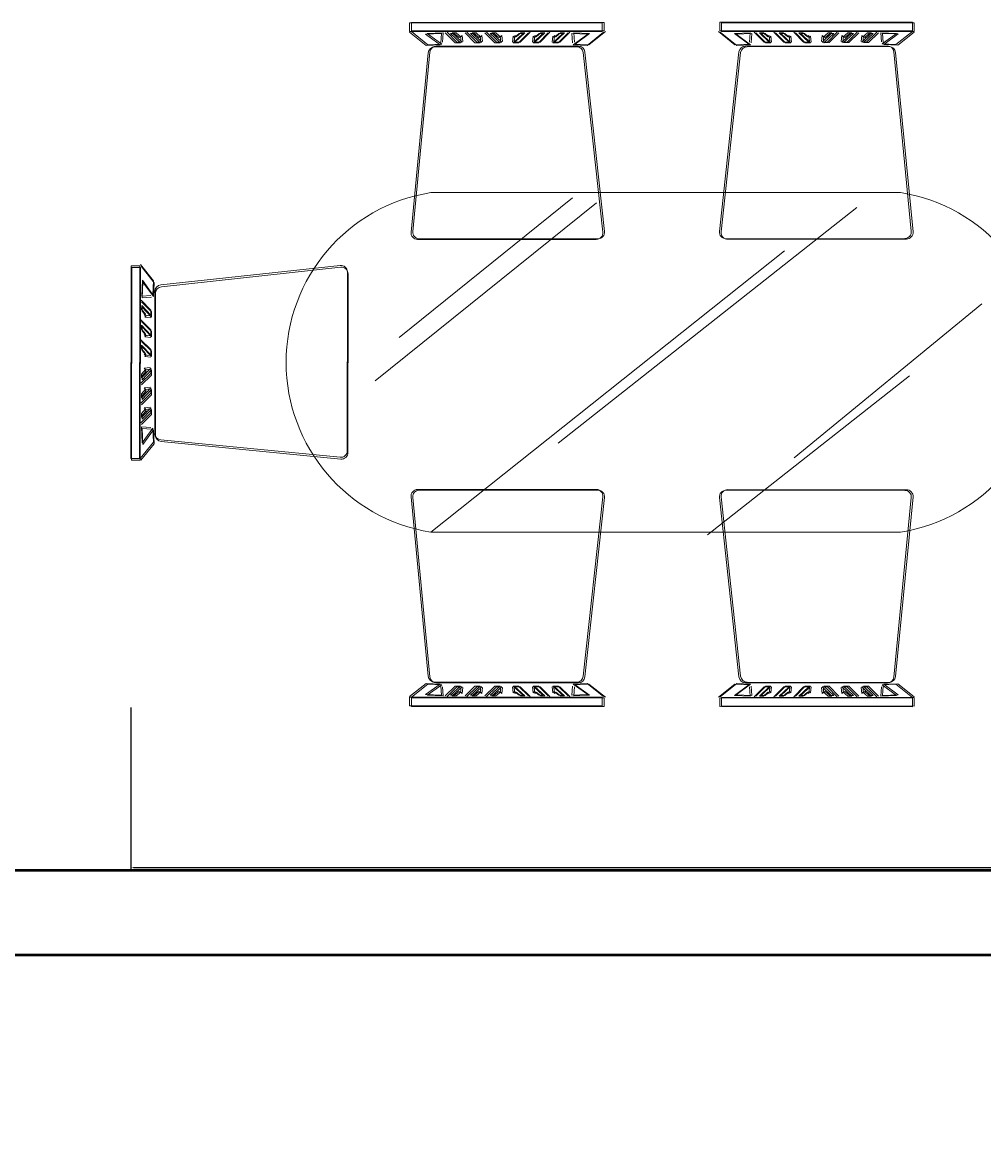
# Model space of a CAD drawing. Units: inches. Extents: x 1305 to 1889, y -508 to -5.
# Tile 4 of 8: x 1403 to 1471, y -303 to -224. Entities that reach past the tile are written whole.
import ezdxf

# ---------------------------------------------------------------- set-up
doc = ezdxf.new("R2010")
doc.units = ezdxf.units.IN
doc.header["$MEASUREMENT"] = 0
for name, color, linetype, lineweight in [('A-ANNO-DIMS', 2, 'Continuous', 18), ('A-FURN', 8, 'Continuous', 18), ('A-WALL', 7, 'Continuous', 50)]:
    doc.layers.add(name, color=color, linetype=linetype, lineweight=lineweight)
doc.styles.get("Standard").update_dxf_attribs({"font": 'arial.ttf', "height": 8})
doc.dimstyles.get("Standard").update_dxf_attribs({"dimtxt": 0.18, "dimasz": 0.18, "dimexe": 0.18, "dimexo": 0.0625, "dimgap": 0.09, "dimtad": 0, "dimtih": 1, "dimtoh": 1, "dimzin": 0, "dimdsep": 46, "dimlunit": 4, "dimtxsty": 'Standard', "dimcen": 0.09, "dimadec": 0, "dimazin": 0, "dimtfac": 1, "dimtofl": 0, "dimtmove": 0, "dimatfit": 3, "dimfxl": 1, "dimtolj": 1, "dimtzin": 0, "dimarcsym": 0})

# ---------------------------------------------------------------- blocks, each defined once
blk = doc.blocks.new('A$C610239F1')
for p, q in [((0.6743, 1.6333, -0.0908), (0.6743, 1.6541, -0.0908)), ((0.6743, 1.6541, -0.0908), (1.1405, 1.6541, -0.0908)), ((0.6785, 1.6349, -0.0908), (0.6785, 1.6556, -0.0908)), ((0.6785, 1.6556, -0.0908), (1.1446, 1.6556, -0.0908)), ((1.1446, 1.6349, -0.0908), (0.6785, 1.6349, -0.0908)), ((1.1405, 1.6541, -0.0908), (1.1405, 1.6333, -0.0908)), ((1.1446, 1.6556, -0.0908), (1.1446, 1.6349, -0.0908)), ((1.8909, 1.6561, -0.0908), (1.4247, 1.6557, -0.0908)), ((1.4247, 1.6557, -0.0908), (1.4247, 1.635, -0.0908)), ((1.4247, 1.635, -0.0908), (1.8909, 1.6354, -0.0908)), ((1.895, 1.6546, -0.0908), (1.4288, 1.6542, -0.0908)), ((1.4288, 1.6542, -0.0908), (1.4289, 1.6335, -0.0908)), ((1.8909, 1.6354, -0.0908), (1.8909, 1.6561, -0.0908)), ((1.895, 1.6339, -0.0908), (1.895, 1.6546, -0.0908)), ((1.1405, 1.6333, -0.0908), (0.6743, 1.6333, -0.0908)), ((0.6743, 1.6317, -0.0908), (0.7143, 1.5998, -0.0908)), ((0.6785, 1.6333, -0.0908), (0.7184, 1.6013, -0.0908)), ((0.7127, 1.627, -0.0908), (0.751, 1.6285, -0.0908)), ((0.7478, 1.6014, -0.0908), (0.7127, 1.627, -0.0908)), ((0.7168, 1.6285, -0.0908), (0.7551, 1.6301, -0.0908)), ((0.7519, 1.6029, -0.0908), (0.7168, 1.6285, -0.0908)), ((0.751, 1.6285, -0.0908), (0.7494, 1.6062, -0.0908)), ((0.7551, 1.6301, -0.0908), (0.7535, 1.6077, -0.0908)), ((0.7606, 1.6301, -0.0908), (0.7845, 1.6062, -0.0908)), ((0.7647, 1.6317, -0.0908), (0.7886, 1.6077, -0.0908)), ((0.7973, 1.6062, -0.0908), (0.7733, 1.6285, -0.0908)), ((0.7733, 1.6285, -0.0908), (0.7829, 1.6285, -0.0908)), ((0.8014, 1.6077, -0.0908), (0.7774, 1.6301, -0.0908)), ((0.7774, 1.6301, -0.0908), (0.787, 1.6301, -0.0908)), ((0.7829, 1.6285, -0.0908), (0.7941, 1.619, -0.0908)), ((0.787, 1.6301, -0.0908), (0.7982, 1.6205, -0.0908)), ((0.7941, 1.619, -0.0908), (0.7973, 1.6222, -0.0908)), ((0.7973, 1.6222, -0.0908), (0.7989, 1.6078, -0.0908)), ((0.7982, 1.6205, -0.0908), (0.8014, 1.6237, -0.0908)), ((0.8014, 1.6237, -0.0908), (0.803, 1.6093, -0.0908)), ((0.8084, 1.6301, -0.0908), (0.8324, 1.6062, -0.0908)), ((0.8126, 1.6317, -0.0908), (0.8365, 1.6077, -0.0908)), ((0.8452, 1.6062, -0.0908), (0.8212, 1.6285, -0.0908)), ((0.8212, 1.6285, -0.0908), (0.8308, 1.6285, -0.0908)), ((0.8493, 1.6077, -0.0908), (0.8253, 1.6301, -0.0908)), ((0.8253, 1.6301, -0.0908), (0.8349, 1.6301, -0.0908)), ((0.8308, 1.6285, -0.0908), (0.842, 1.619, -0.0908)), ((0.8349, 1.6301, -0.0908), (0.8461, 1.6205, -0.0908)), ((0.842, 1.619, -0.0908), (0.8452, 1.6222, -0.0908)), ((0.8452, 1.6222, -0.0908), (0.8468, 1.6078, -0.0908)), ((0.8461, 1.6205, -0.0908), (0.8493, 1.6237, -0.0908)), ((0.8493, 1.6237, -0.0908), (0.8509, 1.6093, -0.0908)), ((0.8563, 1.6301, -0.0908), (0.8803, 1.6062, -0.0908)), ((0.8605, 1.6317, -0.0908), (0.8844, 1.6077, -0.0908)), ((0.8931, 1.6062, -0.0908), (0.8691, 1.6285, -0.0908)), ((0.8691, 1.6285, -0.0908), (0.8787, 1.6285, -0.0908)), ((0.8972, 1.6077, -0.0908), (0.8732, 1.6301, -0.0908)), ((0.8732, 1.6301, -0.0908), (0.8828, 1.6301, -0.0908)), ((0.8787, 1.6285, -0.0908), (0.8899, 1.619, -0.0908)), ((0.8828, 1.6301, -0.0908), (0.894, 1.6205, -0.0908)), ((0.8899, 1.619, -0.0908), (0.8931, 1.6222, -0.0908)), ((0.8931, 1.6222, -0.0908), (0.8947, 1.6078, -0.0908)), ((0.894, 1.6205, -0.0908), (0.8972, 1.6237, -0.0908)), ((0.8972, 1.6237, -0.0908), (0.8988, 1.6093, -0.0908)), ((0.925, 1.6222, -0.0908), (0.9234, 1.6078, -0.0908)), ((0.925, 1.6062, -0.0908), (0.9489, 1.6285, -0.0908)), ((0.9282, 1.619, -0.0908), (0.925, 1.6222, -0.0908)), ((0.9291, 1.6237, -0.0908), (0.9275, 1.6093, -0.0908)), ((0.9394, 1.6285, -0.0908), (0.9282, 1.619, -0.0908)), ((0.9291, 1.6077, -0.0908), (0.9531, 1.6301, -0.0908)), ((0.9323, 1.6205, -0.0908), (0.9291, 1.6237, -0.0908)), ((0.9435, 1.6301, -0.0908), (0.9323, 1.6205, -0.0908)), ((0.9617, 1.6301, -0.0908), (0.9378, 1.6062, -0.0908)), ((0.9489, 1.6285, -0.0908), (0.9394, 1.6285, -0.0908)), ((0.9658, 1.6317, -0.0908), (0.9419, 1.6077, -0.0908)), ((0.9531, 1.6301, -0.0908), (0.9435, 1.6301, -0.0908)), ((0.9729, 1.6222, -0.0908), (0.9713, 1.6078, -0.0908)), ((0.9729, 1.6062, -0.0908), (0.9968, 1.6285, -0.0908)), ((0.9761, 1.619, -0.0908), (0.9729, 1.6222, -0.0908)), ((0.977, 1.6237, -0.0908), (0.9754, 1.6093, -0.0908)), ((0.9873, 1.6285, -0.0908), (0.9761, 1.619, -0.0908)), ((0.977, 1.6077, -0.0908), (1.001, 1.6301, -0.0908)), ((0.9802, 1.6205, -0.0908), (0.977, 1.6237, -0.0908)), ((0.9914, 1.6301, -0.0908), (0.9802, 1.6205, -0.0908)), ((1.0096, 1.6301, -0.0908), (0.9857, 1.6062, -0.0908)), ((0.9968, 1.6285, -0.0908), (0.9873, 1.6285, -0.0908)), ((1.0137, 1.6317, -0.0908), (0.9898, 1.6077, -0.0908)), ((1.001, 1.6301, -0.0908), (0.9914, 1.6301, -0.0908)), ((1.0208, 1.6222, -0.0908), (1.0192, 1.6078, -0.0908)), ((1.0208, 1.6062, -0.0908), (1.0447, 1.6285, -0.0908)), ((1.024, 1.619, -0.0908), (1.0208, 1.6222, -0.0908)), ((1.0249, 1.6237, -0.0908), (1.0233, 1.6093, -0.0908)), ((1.0351, 1.6285, -0.0908), (1.024, 1.619, -0.0908)), ((1.0249, 1.6077, -0.0908), (1.0488, 1.6301, -0.0908)), ((1.0281, 1.6205, -0.0908), (1.0249, 1.6237, -0.0908)), ((1.0393, 1.6301, -0.0908), (1.0281, 1.6205, -0.0908)), ((1.0575, 1.6301, -0.0908), (1.0336, 1.6062, -0.0908)), ((1.0447, 1.6285, -0.0908), (1.0351, 1.6285, -0.0908)), ((1.0616, 1.6317, -0.0908), (1.0377, 1.6077, -0.0908)), ((1.0488, 1.6301, -0.0908), (1.0393, 1.6301, -0.0908)), ((1.1054, 1.627, -0.0908), (1.0671, 1.6285, -0.0908)), ((1.0671, 1.6285, -0.0908), (1.0687, 1.6062, -0.0908)), ((1.0703, 1.6014, -0.0908), (1.1054, 1.627, -0.0908)), ((1.1095, 1.6285, -0.0908), (1.0712, 1.6301, -0.0908)), ((1.0712, 1.6301, -0.0908), (1.0728, 1.6077, -0.0908)), ((1.0744, 1.6029, -0.0908), (1.1095, 1.6285, -0.0908)), ((1.1437, 1.6317, -0.0908), (1.1038, 1.5998, -0.0908)), ((1.1478, 1.6333, -0.0908), (1.1079, 1.6013, -0.0908)), ((1.4216, 1.6334, -0.0908), (1.4615, 1.6015, -0.0908)), ((1.4257, 1.6319, -0.0908), (1.4656, 1.6, -0.0908)), ((1.4289, 1.6335, -0.0908), (1.895, 1.6339, -0.0908)), ((1.4599, 1.6286, -0.0908), (1.4982, 1.6303, -0.0908)), ((1.495, 1.6031, -0.0908), (1.4599, 1.6286, -0.0908)), ((1.464, 1.6271, -0.0908), (1.5023, 1.6287, -0.0908)), ((1.4991, 1.6016, -0.0908), (1.464, 1.6271, -0.0908)), ((1.4982, 1.6303, -0.0908), (1.4966, 1.6079, -0.0908)), ((1.5023, 1.6287, -0.0908), (1.5007, 1.6064, -0.0908)), ((1.5078, 1.6319, -0.0908), (1.5317, 1.6079, -0.0908)), ((1.5119, 1.6303, -0.0908), (1.5359, 1.6064, -0.0908)), ((1.5445, 1.608, -0.0908), (1.5205, 1.6303, -0.0908)), ((1.5205, 1.6303, -0.0908), (1.5301, 1.6303, -0.0908)), ((1.5486, 1.6064, -0.0908), (1.5247, 1.6288, -0.0908)), ((1.5247, 1.6288, -0.0908), (1.5342, 1.6288, -0.0908)), ((1.5301, 1.6303, -0.0908), (1.5413, 1.6207, -0.0908)), ((1.5317, 1.6079, -0.0908), (1.5445, 1.608, -0.0908)), ((1.5342, 1.6288, -0.0908), (1.5454, 1.6192, -0.0908)), ((1.5413, 1.6207, -0.0908), (1.5445, 1.6239, -0.0908)), ((1.5445, 1.6239, -0.0908), (1.5461, 1.6095, -0.0908)), ((1.5454, 1.6192, -0.0908), (1.5486, 1.6224, -0.0908)), ((1.5486, 1.6224, -0.0908), (1.5502, 1.608, -0.0908)), ((1.5557, 1.6319, -0.0908), (1.5796, 1.608, -0.0908)), ((1.5598, 1.6304, -0.0908), (1.5837, 1.6065, -0.0908)), ((1.5924, 1.608, -0.0908), (1.5684, 1.6303, -0.0908)), ((1.5684, 1.6303, -0.0908), (1.578, 1.6303, -0.0908)), ((1.5965, 1.6065, -0.0908), (1.5726, 1.6288, -0.0908)), ((1.5726, 1.6288, -0.0908), (1.5821, 1.6288, -0.0908)), ((1.578, 1.6303, -0.0908), (1.5892, 1.6208, -0.0908)), ((1.5796, 1.608, -0.0908), (1.5924, 1.608, -0.0908)), ((1.5821, 1.6288, -0.0908), (1.5933, 1.6192, -0.0908)), ((1.5892, 1.6208, -0.0908), (1.5924, 1.624, -0.0908)), ((1.5924, 1.624, -0.0908), (1.594, 1.6096, -0.0908)), ((1.5933, 1.6192, -0.0908), (1.5965, 1.6224, -0.0908)), ((1.5965, 1.6224, -0.0908), (1.5981, 1.6081, -0.0908)), ((1.6036, 1.6319, -0.0908), (1.6275, 1.608, -0.0908)), ((1.6077, 1.6304, -0.0908), (1.6316, 1.6065, -0.0908)), ((1.6403, 1.608, -0.0908), (1.6163, 1.6304, -0.0908)), ((1.6163, 1.6304, -0.0908), (1.6259, 1.6304, -0.0908)), ((1.6444, 1.6065, -0.0908), (1.6204, 1.6288, -0.0908)), ((1.6204, 1.6288, -0.0908), (1.63, 1.6288, -0.0908)), ((1.6259, 1.6304, -0.0908), (1.6371, 1.6208, -0.0908)), ((1.6275, 1.608, -0.0908), (1.6403, 1.608, -0.0908)), ((1.63, 1.6288, -0.0908), (1.6412, 1.6193, -0.0908)), ((1.6371, 1.6208, -0.0908), (1.6403, 1.624, -0.0908)), ((1.6403, 1.624, -0.0908), (1.6419, 1.6096, -0.0908)), ((1.6412, 1.6193, -0.0908), (1.6444, 1.6225, -0.0908)), ((1.6444, 1.6225, -0.0908), (1.646, 1.6081, -0.0908)), ((1.6722, 1.624, -0.0908), (1.6706, 1.6097, -0.0908)), ((1.6722, 1.6081, -0.0908), (1.6962, 1.6304, -0.0908)), ((1.6754, 1.6208, -0.0908), (1.6722, 1.624, -0.0908)), ((1.685, 1.6081, -0.0908), (1.6722, 1.6081, -0.0908)), ((1.6763, 1.6225, -0.0908), (1.6747, 1.6081, -0.0908)), ((1.6866, 1.6304, -0.0908), (1.6754, 1.6208, -0.0908)), ((1.6763, 1.6065, -0.0908), (1.7003, 1.6289, -0.0908)), ((1.6795, 1.6193, -0.0908), (1.6763, 1.6225, -0.0908)), ((1.6907, 1.6289, -0.0908), (1.6795, 1.6193, -0.0908)), ((1.7089, 1.632, -0.0908), (1.685, 1.6081, -0.0908)), ((1.6962, 1.6304, -0.0908), (1.6866, 1.6304, -0.0908)), ((1.713, 1.6305, -0.0908), (1.6891, 1.6066, -0.0908)), ((1.7003, 1.6289, -0.0908), (1.6907, 1.6289, -0.0908)), ((1.7201, 1.6241, -0.0908), (1.7185, 1.6097, -0.0908)), ((1.7201, 1.6081, -0.0908), (1.744, 1.6305, -0.0908)), ((1.7233, 1.6209, -0.0908), (1.7201, 1.6241, -0.0908)), ((1.7329, 1.6081, -0.0908), (1.7201, 1.6081, -0.0908)), ((1.7242, 1.6225, -0.0908), (1.7226, 1.6082, -0.0908)), ((1.7345, 1.6305, -0.0908), (1.7233, 1.6209, -0.0908)), ((1.7242, 1.6066, -0.0908), (1.7482, 1.629, -0.0908)), ((1.7274, 1.6194, -0.0908), (1.7242, 1.6225, -0.0908)), ((1.7386, 1.6289, -0.0908), (1.7274, 1.6194, -0.0908)), ((1.7568, 1.6321, -0.0908), (1.7329, 1.6081, -0.0908)), ((1.744, 1.6305, -0.0908), (1.7345, 1.6305, -0.0908)), ((1.7609, 1.6306, -0.0908), (1.737, 1.6066, -0.0908)), ((1.7482, 1.629, -0.0908), (1.7386, 1.6289, -0.0908)), ((1.768, 1.6241, -0.0908), (1.7664, 1.6097, -0.0908)), ((1.768, 1.6081, -0.0908), (1.7919, 1.6305, -0.0908)), ((1.7712, 1.6209, -0.0908), (1.768, 1.6241, -0.0908)), ((1.7808, 1.6082, -0.0908), (1.768, 1.6081, -0.0908)), ((1.7721, 1.6226, -0.0908), (1.7705, 1.6082, -0.0908)), ((1.7824, 1.6305, -0.0908), (1.7712, 1.6209, -0.0908)), ((1.7721, 1.6066, -0.0908), (1.7961, 1.629, -0.0908)), ((1.7753, 1.6194, -0.0908), (1.7721, 1.6226, -0.0908)), ((1.7865, 1.629, -0.0908), (1.7753, 1.6194, -0.0908)), ((1.8047, 1.6321, -0.0908), (1.7808, 1.6082, -0.0908)), ((1.7919, 1.6305, -0.0908), (1.7824, 1.6305, -0.0908)), ((1.8088, 1.6306, -0.0908), (1.7849, 1.6066, -0.0908)), ((1.7961, 1.629, -0.0908), (1.7865, 1.629, -0.0908)), ((1.8526, 1.629, -0.0908), (1.8143, 1.6305, -0.0908)), ((1.8143, 1.6305, -0.0908), (1.8159, 1.6082, -0.0908)), ((1.8175, 1.6034, -0.0908), (1.8526, 1.629, -0.0908)), ((1.8567, 1.6275, -0.0908), (1.8184, 1.629, -0.0908)), ((1.8184, 1.629, -0.0908), (1.82, 1.6067, -0.0908)), ((1.8216, 1.6019, -0.0908), (1.8567, 1.6275, -0.0908)), ((1.8909, 1.6338, -0.0908), (1.851, 1.6018, -0.0908)), ((1.895, 1.6323, -0.0908), (1.8552, 1.6003, -0.0908)), ((0.7193, 1.5822, -0.0908), (0.6776, 1.1482, -0.0908)), ((0.7234, 1.5837, -0.0908), (0.6817, 1.1497, -0.0908)), ((0.7143, 1.5998, -0.0908), (0.7478, 1.6014, -0.0908)), ((0.7184, 1.6013, -0.0908), (0.7519, 1.6029, -0.0908)), ((1.0783, 1.5966, -0.0908), (0.7351, 1.5966, -0.0908)), ((1.0824, 1.5981, -0.0908), (0.7393, 1.5981, -0.0908)), ((0.7845, 1.6062, -0.0908), (0.7973, 1.6062, -0.0908)), ((0.7886, 1.6077, -0.0908), (0.8014, 1.6077, -0.0908)), ((0.8324, 1.6062, -0.0908), (0.8452, 1.6062, -0.0908)), ((0.8365, 1.6077, -0.0908), (0.8493, 1.6077, -0.0908)), ((0.8803, 1.6062, -0.0908), (0.8931, 1.6062, -0.0908)), ((0.8844, 1.6077, -0.0908), (0.8972, 1.6077, -0.0908)), ((0.9378, 1.6062, -0.0908), (0.925, 1.6062, -0.0908)), ((0.9419, 1.6077, -0.0908), (0.9291, 1.6077, -0.0908)), ((0.9857, 1.6062, -0.0908), (0.9729, 1.6062, -0.0908)), ((0.9898, 1.6077, -0.0908), (0.977, 1.6077, -0.0908)), ((1.0336, 1.6062, -0.0908), (1.0208, 1.6062, -0.0908)), ((1.0377, 1.6077, -0.0908), (1.0249, 1.6077, -0.0908)), ((1.1038, 1.5998, -0.0908), (1.0703, 1.6014, -0.0908)), ((1.1079, 1.6013, -0.0908), (1.0744, 1.6029, -0.0908)), ((1.1418, 1.1484, -0.0908), (1.0942, 1.5824, -0.0908)), ((1.1459, 1.1499, -0.0908), (1.0983, 1.5839, -0.0908)), ((1.4239, 1.15, -0.0908), (1.4711, 1.5841, -0.0908)), ((1.428, 1.1485, -0.0908), (1.4752, 1.5826, -0.0908)), ((1.4615, 1.6015, -0.0908), (1.495, 1.6031, -0.0908)), ((1.4656, 1.6, -0.0908), (1.4991, 1.6016, -0.0908)), ((1.487, 1.5983, -0.0908), (1.8301, 1.5986, -0.0908)), ((1.4911, 1.5968, -0.0908), (1.8343, 1.5971, -0.0908)), ((1.5359, 1.6064, -0.0908), (1.5486, 1.6064, -0.0908)), ((1.5837, 1.6065, -0.0908), (1.5965, 1.6065, -0.0908)), ((1.6316, 1.6065, -0.0908), (1.6444, 1.6065, -0.0908)), ((1.6891, 1.6066, -0.0908), (1.6763, 1.6065, -0.0908)), ((1.737, 1.6066, -0.0908), (1.7242, 1.6066, -0.0908)), ((1.7849, 1.6066, -0.0908), (1.7721, 1.6066, -0.0908)), ((1.851, 1.6018, -0.0908), (1.8175, 1.6034, -0.0908)), ((1.8552, 1.6003, -0.0908), (1.8216, 1.6019, -0.0908)), ((1.8461, 1.5842, -0.0908), (1.8881, 1.1502, -0.0908)), ((1.8502, 1.5827, -0.0908), (1.8922, 1.1487, -0.0908)), ((1.8623, 1.2439), (0.7253, 1.2439)), ((0.5907, 0.7886), (1.1267, 1.2192)), ((0.6489, 0.8934), (1.0684, 1.2309)), ((1.0335, 0.6373), (1.7559, 1.2076)), ((0.6935, 1.1307, -0.0908), (1.1259, 1.1307, -0.0908)), ((0.6976, 1.1322, -0.0908), (1.13, 1.1322, -0.0908)), ((1.8722, 1.1327, -0.0908), (1.4398, 1.1323, -0.0908)), ((1.8763, 1.1312, -0.0908), (1.4439, 1.1308, -0.0908)), ((0.7253, 0.4224), (1.5811, 1.1029)), ((0, 0.6006, -0.0908), (0.0004, 1.0667, -0.0908)), ((0.0004, 1.0667, -0.0908), (0.0212, 1.0667, -0.0908)), ((0.0015, 0.5964, -0.0908), (0.0019, 1.0626, -0.0908)), ((0.0019, 1.0626, -0.0908), (0.0227, 1.0626, -0.0908)), ((0.0212, 1.0667, -0.0908), (0.0207, 0.6005, -0.0908)), ((0.0227, 1.0626, -0.0908), (0.0223, 0.5964, -0.0908)), ((0.0228, 1.0699, -0.0908), (0.0546, 1.03, -0.0908)), ((0.0243, 1.0658, -0.0908), (0.0561, 1.0258, -0.0908)), ((0.5061, 1.0675, -0.0908), (0.072, 1.0203, -0.0908)), ((0.5076, 1.0634, -0.0908), (0.0736, 1.0162, -0.0908)), ((0.5234, 0.6193, -0.0908), (0.5238, 1.0517, -0.0908)), ((0.5249, 0.6151, -0.0908), (0.5253, 1.0475, -0.0908)), ((0.0275, 1.0316, -0.0908), (0.0259, 0.9933, -0.0908)), ((0.029, 1.0275, -0.0908), (0.0274, 0.9892, -0.0908)), ((0.053, 0.9964, -0.0908), (0.0275, 1.0316, -0.0908)), ((0.0545, 0.9923, -0.0908), (0.029, 1.0275, -0.0908)), ((0.0546, 1.03, -0.0908), (0.053, 0.9964, -0.0908)), ((0.0561, 1.0258, -0.0908), (0.0545, 0.9923, -0.0908)), ((0.0259, 0.9933, -0.0908), (0.0482, 0.9948, -0.0908)), ((0.0578, 1.0045, -0.0908), (0.0575, 0.6613, -0.0908)), ((0.0593, 1.0004, -0.0908), (0.059, 0.6572, -0.0908)), ((0.0243, 0.9837, -0.0908), (0.0482, 0.9597, -0.0908)), ((0.0258, 0.9796, -0.0908), (0.0497, 0.9556, -0.0908)), ((0.0259, 0.9709, -0.0908), (0.0258, 0.9613, -0.0908)), ((0.0482, 0.947, -0.0908), (0.0259, 0.9709, -0.0908)), ((0.0274, 0.9892, -0.0908), (0.0497, 0.9907, -0.0908)), ((0.0497, 0.9428, -0.0908), (0.0274, 0.9668, -0.0908)), ((0.0274, 0.9668, -0.0908), (0.0274, 0.9572, -0.0908)), ((1.6044, 0.6024), (2.0589, 0.9748)), ((0.0258, 0.9613, -0.0908), (0.0354, 0.9502, -0.0908)), ((0.0274, 0.9572, -0.0908), (0.0369, 0.946, -0.0908)), ((0.0354, 0.9502, -0.0908), (0.0322, 0.947, -0.0908)), ((0.0322, 0.947, -0.0908), (0.0466, 0.9454, -0.0908)), ((0.0369, 0.946, -0.0908), (0.0337, 0.9428, -0.0908)), ((0.0337, 0.9428, -0.0908), (0.0481, 0.9412, -0.0908)), ((0.0482, 0.9597, -0.0908), (0.0482, 0.947, -0.0908)), ((0.0497, 0.9556, -0.0908), (0.0497, 0.9428, -0.0908)), ((0.0242, 0.9358, -0.0908), (0.0481, 0.9118, -0.0908)), ((0.0257, 0.9317, -0.0908), (0.0497, 0.9077, -0.0908)), ((0.0481, 0.8991, -0.0908), (0.0258, 0.923, -0.0908)), ((0.0258, 0.923, -0.0908), (0.0258, 0.9134, -0.0908)), ((0.0258, 0.9134, -0.0908), (0.0354, 0.9023, -0.0908)), ((0.0496, 0.8949, -0.0908), (0.0273, 0.9189, -0.0908)), ((0.0273, 0.9189, -0.0908), (0.0273, 0.9093, -0.0908)), ((0.0481, 0.9118, -0.0908), (0.0481, 0.8991, -0.0908)), ((0.0242, 0.8879, -0.0908), (0.0481, 0.8639, -0.0908)), ((0.0273, 0.9093, -0.0908), (0.0369, 0.8981, -0.0908)), ((0.0354, 0.9023, -0.0908), (0.0322, 0.8991, -0.0908)), ((0.0322, 0.8991, -0.0908), (0.0465, 0.8975, -0.0908)), ((0.0369, 0.8981, -0.0908), (0.0337, 0.895, -0.0908)), ((0.0337, 0.895, -0.0908), (0.048, 0.8933, -0.0908)), ((0.0497, 0.9077, -0.0908), (0.0496, 0.8949, -0.0908)), ((0.0257, 0.8838, -0.0908), (0.0496, 0.8598, -0.0908)), ((0.0481, 0.8512, -0.0908), (0.0258, 0.8751, -0.0908)), ((0.0258, 0.8751, -0.0908), (0.0258, 0.8656, -0.0908)), ((0.0258, 0.8656, -0.0908), (0.0353, 0.8544, -0.0908)), ((0.0496, 0.847, -0.0908), (0.0273, 0.871, -0.0908)), ((0.0273, 0.871, -0.0908), (0.0273, 0.8614, -0.0908)), ((0.0273, 0.8614, -0.0908), (0.0368, 0.8502, -0.0908)), ((0.0481, 0.8639, -0.0908), (0.0481, 0.8512, -0.0908)), ((0.0496, 0.8598, -0.0908), (0.0496, 0.847, -0.0908)), ((0.0353, 0.8544, -0.0908), (0.0321, 0.8512, -0.0908)), ((0.0321, 0.8512, -0.0908), (0.0465, 0.8496, -0.0908)), ((0.0368, 0.8502, -0.0908), (0.0336, 0.8471, -0.0908)), ((0.0336, 0.8471, -0.0908), (0.048, 0.8454, -0.0908)), ((0.0241, 0.7825, -0.0908), (0.0481, 0.8065, -0.0908)), ((0.0481, 0.8192, -0.0908), (0.0257, 0.7953, -0.0908)), ((0.0257, 0.8049, -0.0908), (0.0353, 0.8161, -0.0908)), ((0.0257, 0.7953, -0.0908), (0.0257, 0.8049, -0.0908)), ((0.0496, 0.8151, -0.0908), (0.0272, 0.7912, -0.0908)), ((0.0272, 0.8008, -0.0908), (0.0368, 0.8119, -0.0908)), ((0.0321, 0.8192, -0.0908), (0.0465, 0.8208, -0.0908)), ((0.0353, 0.8161, -0.0908), (0.0321, 0.8192, -0.0908)), ((0.0336, 0.8151, -0.0908), (0.048, 0.8167, -0.0908)), ((0.0368, 0.8119, -0.0908), (0.0336, 0.8151, -0.0908)), ((0.0481, 0.8065, -0.0908), (0.0481, 0.8192, -0.0908)), ((0.0496, 0.8023, -0.0908), (0.0496, 0.8151, -0.0908)), ((0.0256, 0.7784, -0.0908), (0.0496, 0.8023, -0.0908)), ((0.0272, 0.7912, -0.0908), (0.0272, 0.8008, -0.0908)), ((1.3947, 0.4162), (1.8841, 0.8002)), ((0.0241, 0.7346, -0.0908), (0.048, 0.7586, -0.0908)), ((0.0256, 0.7305, -0.0908), (0.0495, 0.7544, -0.0908)), ((0.048, 0.7713, -0.0908), (0.0257, 0.7474, -0.0908)), ((0.0257, 0.757, -0.0908), (0.0353, 0.7682, -0.0908)), ((0.0257, 0.7474, -0.0908), (0.0257, 0.757, -0.0908)), ((0.0495, 0.7672, -0.0908), (0.0272, 0.7433, -0.0908)), ((0.0272, 0.7529, -0.0908), (0.0368, 0.764, -0.0908)), ((0.0272, 0.7433, -0.0908), (0.0272, 0.7529, -0.0908)), ((0.0321, 0.7714, -0.0908), (0.0464, 0.7729, -0.0908)), ((0.0353, 0.7682, -0.0908), (0.0321, 0.7714, -0.0908)), ((0.0336, 0.7672, -0.0908), (0.0479, 0.7688, -0.0908)), ((0.0368, 0.764, -0.0908), (0.0336, 0.7672, -0.0908)), ((0.048, 0.7586, -0.0908), (0.048, 0.7713, -0.0908)), ((0.0495, 0.7544, -0.0908), (0.0495, 0.7672, -0.0908)), ((0.032, 0.7235, -0.0908), (0.0464, 0.725, -0.0908)), ((0.024, 0.6867, -0.0908), (0.048, 0.7107, -0.0908)), ((0.0255, 0.6826, -0.0908), (0.0495, 0.7066, -0.0908)), ((0.048, 0.7234, -0.0908), (0.0256, 0.6995, -0.0908)), ((0.0256, 0.7091, -0.0908), (0.0352, 0.7203, -0.0908)), ((0.0256, 0.6995, -0.0908), (0.0256, 0.7091, -0.0908)), ((0.0495, 0.7193, -0.0908), (0.0271, 0.6954, -0.0908)), ((0.0271, 0.705, -0.0908), (0.0367, 0.7161, -0.0908)), ((0.0271, 0.6954, -0.0908), (0.0271, 0.705, -0.0908)), ((0.0352, 0.7203, -0.0908), (0.032, 0.7235, -0.0908)), ((0.0335, 0.7193, -0.0908), (0.0479, 0.7209, -0.0908)), ((0.0367, 0.7161, -0.0908), (0.0335, 0.7193, -0.0908)), ((0.048, 0.7107, -0.0908), (0.048, 0.7234, -0.0908)), ((0.0495, 0.7066, -0.0908), (0.0495, 0.7193, -0.0908)), ((0.0272, 0.6388, -0.0908), (0.0256, 0.6772, -0.0908)), ((0.0256, 0.6772, -0.0908), (0.0479, 0.6755, -0.0908)), ((0.0287, 0.6347, -0.0908), (0.0271, 0.673, -0.0908)), ((0.0271, 0.673, -0.0908), (0.0495, 0.6714, -0.0908)), ((0.0527, 0.6739, -0.0908), (0.0272, 0.6388, -0.0908)), ((0.0543, 0.6404, -0.0908), (0.0527, 0.6739, -0.0908)), ((0.0542, 0.6698, -0.0908), (0.0287, 0.6347, -0.0908)), ((0.0558, 0.6363, -0.0908), (0.0542, 0.6698, -0.0908)), ((0.0719, 0.6454, -0.0908), (0.5059, 0.6034, -0.0908)), ((0.0223, 0.6005, -0.0908), (0.0543, 0.6404, -0.0908)), ((0.0239, 0.5964, -0.0908), (0.0558, 0.6363, -0.0908)), ((0.0734, 0.6413, -0.0908), (0.5074, 0.5993, -0.0908)), ((0.0207, 0.6005, -0.0908), (0, 0.6006, -0.0908)), ((0.0223, 0.5964, -0.0908), (0.0015, 0.5964, -0.0908)), ((0.6935, 0.5254, -0.0908), (1.1259, 0.5254, -0.0908)), ((0.6976, 0.5239, -0.0908), (1.13, 0.5239, -0.0908)), ((1.8722, 0.5234, -0.0908), (1.4398, 0.5238, -0.0908)), ((1.8763, 0.5249, -0.0908), (1.4439, 0.5253, -0.0908)), ((0.7193, 0.0739, -0.0908), (0.6776, 0.5079, -0.0908)), ((0.7234, 0.0724, -0.0908), (0.6817, 0.5064, -0.0908)), ((1.1418, 0.5077, -0.0908), (1.0942, 0.0737, -0.0908)), ((1.1459, 0.5062, -0.0908), (1.0983, 0.0722, -0.0908)), ((1.4239, 0.5061, -0.0908), (1.4711, 0.072, -0.0908)), ((1.428, 0.5076, -0.0908), (1.4752, 0.0736, -0.0908)), ((1.8461, 0.0719, -0.0908), (1.8881, 0.5059, -0.0908)), ((1.8502, 0.0734, -0.0908), (1.8922, 0.5074, -0.0908)), ((0.7253, 0.4224), (1.8623, 0.4224)), ((0.6743, 0.0244, -0.0908), (0.7143, 0.0563, -0.0908)), ((0.6785, 0.0229, -0.0908), (0.7184, 0.0548, -0.0908)), ((0.7478, 0.0547, -0.0908), (0.7127, 0.0292, -0.0908)), ((0.7143, 0.0563, -0.0908), (0.7478, 0.0547, -0.0908)), ((0.7184, 0.0548, -0.0908), (0.7519, 0.0532, -0.0908)), ((1.0783, 0.0595, -0.0908), (0.7351, 0.0595, -0.0908)), ((1.0824, 0.058, -0.0908), (0.7393, 0.058, -0.0908)), ((1.1038, 0.0563, -0.0908), (1.0703, 0.0547, -0.0908)), ((1.0703, 0.0547, -0.0908), (1.1054, 0.0292, -0.0908)), ((1.1079, 0.0548, -0.0908), (1.0744, 0.0532, -0.0908)), ((1.1437, 0.0244, -0.0908), (1.1038, 0.0563, -0.0908)), ((1.1478, 0.0229, -0.0908), (1.1079, 0.0548, -0.0908)), ((1.4216, 0.0228, -0.0908), (1.4615, 0.0546, -0.0908)), ((1.4257, 0.0243, -0.0908), (1.4656, 0.0561, -0.0908)), ((1.4615, 0.0546, -0.0908), (1.495, 0.053, -0.0908)), ((1.4991, 0.0545, -0.0908), (1.464, 0.029, -0.0908)), ((1.4656, 0.0561, -0.0908), (1.4991, 0.0545, -0.0908)), ((1.487, 0.0578, -0.0908), (1.8301, 0.0575, -0.0908)), ((1.4911, 0.0593, -0.0908), (1.8343, 0.059, -0.0908)), ((1.851, 0.0543, -0.0908), (1.8175, 0.0527, -0.0908)), ((1.8552, 0.0558, -0.0908), (1.8216, 0.0542, -0.0908)), ((1.8216, 0.0542, -0.0908), (1.8567, 0.0287, -0.0908)), ((1.8909, 0.0223, -0.0908), (1.851, 0.0543, -0.0908)), ((1.895, 0.0239, -0.0908), (1.8552, 0.0558, -0.0908)), ((0.7127, 0.0292, -0.0908), (0.751, 0.0276, -0.0908)), ((0.7519, 0.0532, -0.0908), (0.7168, 0.0277, -0.0908)), ((0.7168, 0.0277, -0.0908), (0.7551, 0.0261, -0.0908)), ((0.751, 0.0276, -0.0908), (0.7494, 0.0499, -0.0908)), ((0.7551, 0.0261, -0.0908), (0.7535, 0.0484, -0.0908)), ((0.7606, 0.026, -0.0908), (0.7845, 0.0499, -0.0908)), ((0.7647, 0.0245, -0.0908), (0.7886, 0.0484, -0.0908)), ((0.7973, 0.0499, -0.0908), (0.7733, 0.0276, -0.0908)), ((0.7733, 0.0276, -0.0908), (0.7829, 0.0276, -0.0908)), ((0.8014, 0.0484, -0.0908), (0.7774, 0.0261, -0.0908)), ((0.7829, 0.0276, -0.0908), (0.7941, 0.0372, -0.0908)), ((0.7845, 0.0499, -0.0908), (0.7973, 0.0499, -0.0908)), ((0.787, 0.0261, -0.0908), (0.7982, 0.0356, -0.0908)), ((0.7886, 0.0484, -0.0908), (0.8014, 0.0484, -0.0908)), ((0.7941, 0.0372, -0.0908), (0.7973, 0.034, -0.0908)), ((0.7973, 0.034, -0.0908), (0.7989, 0.0483, -0.0908)), ((0.7982, 0.0356, -0.0908), (0.8014, 0.0324, -0.0908)), ((0.8014, 0.0324, -0.0908), (0.803, 0.0468, -0.0908)), ((0.8084, 0.026, -0.0908), (0.8324, 0.0499, -0.0908)), ((0.8126, 0.0245, -0.0908), (0.8365, 0.0484, -0.0908)), ((0.8452, 0.0499, -0.0908), (0.8212, 0.0276, -0.0908)), ((0.8212, 0.0276, -0.0908), (0.8308, 0.0276, -0.0908)), ((0.8493, 0.0484, -0.0908), (0.8253, 0.0261, -0.0908)), ((0.8308, 0.0276, -0.0908), (0.842, 0.0372, -0.0908)), ((0.8324, 0.0499, -0.0908), (0.8452, 0.0499, -0.0908)), ((0.8349, 0.0261, -0.0908), (0.8461, 0.0356, -0.0908)), ((0.8365, 0.0484, -0.0908), (0.8493, 0.0484, -0.0908)), ((0.842, 0.0372, -0.0908), (0.8452, 0.034, -0.0908)), ((0.8452, 0.034, -0.0908), (0.8468, 0.0483, -0.0908)), ((0.8461, 0.0356, -0.0908), (0.8493, 0.0324, -0.0908)), ((0.8493, 0.0324, -0.0908), (0.8509, 0.0468, -0.0908)), ((0.8563, 0.026, -0.0908), (0.8803, 0.0499, -0.0908)), ((0.8605, 0.0245, -0.0908), (0.8844, 0.0484, -0.0908)), ((0.8931, 0.0499, -0.0908), (0.8691, 0.0276, -0.0908)), ((0.8691, 0.0276, -0.0908), (0.8787, 0.0276, -0.0908)), ((0.8972, 0.0484, -0.0908), (0.8732, 0.0261, -0.0908)), ((0.8787, 0.0276, -0.0908), (0.8899, 0.0372, -0.0908)), ((0.8803, 0.0499, -0.0908), (0.8931, 0.0499, -0.0908)), ((0.8828, 0.0261, -0.0908), (0.894, 0.0356, -0.0908)), ((0.8844, 0.0484, -0.0908), (0.8972, 0.0484, -0.0908)), ((0.8899, 0.0372, -0.0908), (0.8931, 0.034, -0.0908)), ((0.8931, 0.034, -0.0908), (0.8947, 0.0483, -0.0908)), ((0.894, 0.0356, -0.0908), (0.8972, 0.0324, -0.0908)), ((0.8972, 0.0324, -0.0908), (0.8988, 0.0468, -0.0908)), ((0.925, 0.034, -0.0908), (0.9234, 0.0483, -0.0908)), ((0.9378, 0.0499, -0.0908), (0.925, 0.0499, -0.0908)), ((0.925, 0.0499, -0.0908), (0.9489, 0.0276, -0.0908)), ((0.9282, 0.0372, -0.0908), (0.925, 0.034, -0.0908)), ((0.9291, 0.0324, -0.0908), (0.9275, 0.0468, -0.0908)), ((0.9394, 0.0276, -0.0908), (0.9282, 0.0372, -0.0908)), ((0.9419, 0.0484, -0.0908), (0.9291, 0.0484, -0.0908)), ((0.9291, 0.0484, -0.0908), (0.9531, 0.0261, -0.0908)), ((0.9323, 0.0356, -0.0908), (0.9291, 0.0324, -0.0908)), ((0.9435, 0.0261, -0.0908), (0.9323, 0.0356, -0.0908)), ((0.9617, 0.026, -0.0908), (0.9378, 0.0499, -0.0908)), ((0.9489, 0.0276, -0.0908), (0.9394, 0.0276, -0.0908)), ((0.9658, 0.0245, -0.0908), (0.9419, 0.0484, -0.0908)), ((0.9729, 0.034, -0.0908), (0.9713, 0.0483, -0.0908)), ((0.9857, 0.0499, -0.0908), (0.9729, 0.0499, -0.0908)), ((0.9729, 0.0499, -0.0908), (0.9968, 0.0276, -0.0908)), ((0.9761, 0.0372, -0.0908), (0.9729, 0.034, -0.0908)), ((0.977, 0.0324, -0.0908), (0.9754, 0.0468, -0.0908)), ((0.9873, 0.0276, -0.0908), (0.9761, 0.0372, -0.0908)), ((0.9898, 0.0484, -0.0908), (0.977, 0.0484, -0.0908)), ((0.977, 0.0484, -0.0908), (1.001, 0.0261, -0.0908)), ((0.9802, 0.0356, -0.0908), (0.977, 0.0324, -0.0908)), ((0.9914, 0.0261, -0.0908), (0.9802, 0.0356, -0.0908)), ((1.0096, 0.026, -0.0908), (0.9857, 0.0499, -0.0908)), ((0.9968, 0.0276, -0.0908), (0.9873, 0.0276, -0.0908)), ((1.0137, 0.0245, -0.0908), (0.9898, 0.0484, -0.0908)), ((1.0208, 0.034, -0.0908), (1.0192, 0.0483, -0.0908)), ((1.0336, 0.0499, -0.0908), (1.0208, 0.0499, -0.0908)), ((1.0208, 0.0499, -0.0908), (1.0447, 0.0276, -0.0908)), ((1.024, 0.0372, -0.0908), (1.0208, 0.034, -0.0908)), ((1.0249, 0.0324, -0.0908), (1.0233, 0.0468, -0.0908)), ((1.0351, 0.0276, -0.0908), (1.024, 0.0372, -0.0908)), ((1.0377, 0.0484, -0.0908), (1.0249, 0.0484, -0.0908)), ((1.0249, 0.0484, -0.0908), (1.0488, 0.0261, -0.0908)), ((1.0281, 0.0356, -0.0908), (1.0249, 0.0324, -0.0908)), ((1.0393, 0.0261, -0.0908), (1.0281, 0.0356, -0.0908)), ((1.0575, 0.026, -0.0908), (1.0336, 0.0499, -0.0908)), ((1.0447, 0.0276, -0.0908), (1.0351, 0.0276, -0.0908)), ((1.0616, 0.0245, -0.0908), (1.0377, 0.0484, -0.0908)), ((1.0671, 0.0276, -0.0908), (1.0687, 0.0499, -0.0908)), ((1.1054, 0.0292, -0.0908), (1.0671, 0.0276, -0.0908)), ((1.0712, 0.0261, -0.0908), (1.0728, 0.0484, -0.0908)), ((1.1095, 0.0277, -0.0908), (1.0712, 0.0261, -0.0908)), ((1.0744, 0.0532, -0.0908), (1.1095, 0.0277, -0.0908)), ((1.495, 0.053, -0.0908), (1.4599, 0.0275, -0.0908)), ((1.4599, 0.0275, -0.0908), (1.4982, 0.0259, -0.0908)), ((1.464, 0.029, -0.0908), (1.5023, 0.0274, -0.0908)), ((1.4982, 0.0259, -0.0908), (1.4966, 0.0482, -0.0908)), ((1.5023, 0.0274, -0.0908), (1.5007, 0.0497, -0.0908)), ((1.5078, 0.0243, -0.0908), (1.5317, 0.0482, -0.0908)), ((1.5119, 0.0258, -0.0908), (1.5359, 0.0497, -0.0908)), ((1.5445, 0.0482, -0.0908), (1.5205, 0.0259, -0.0908)), ((1.5486, 0.0497, -0.0908), (1.5247, 0.0274, -0.0908)), ((1.5247, 0.0274, -0.0908), (1.5342, 0.0274, -0.0908)), ((1.5301, 0.0258, -0.0908), (1.5413, 0.0354, -0.0908)), ((1.5317, 0.0482, -0.0908), (1.5445, 0.0482, -0.0908)), ((1.5342, 0.0274, -0.0908), (1.5454, 0.0369, -0.0908)), ((1.5359, 0.0497, -0.0908), (1.5486, 0.0497, -0.0908)), ((1.5413, 0.0354, -0.0908), (1.5445, 0.0322, -0.0908)), ((1.5445, 0.0322, -0.0908), (1.5461, 0.0466, -0.0908)), ((1.5454, 0.0369, -0.0908), (1.5486, 0.0337, -0.0908)), ((1.5486, 0.0337, -0.0908), (1.5502, 0.0481, -0.0908)), ((1.5557, 0.0242, -0.0908), (1.5796, 0.0481, -0.0908)), ((1.5598, 0.0257, -0.0908), (1.5837, 0.0497, -0.0908)), ((1.5924, 0.0481, -0.0908), (1.5684, 0.0258, -0.0908)), ((1.5965, 0.0496, -0.0908), (1.5726, 0.0273, -0.0908)), ((1.5726, 0.0273, -0.0908), (1.5821, 0.0273, -0.0908)), ((1.578, 0.0258, -0.0908), (1.5892, 0.0354, -0.0908)), ((1.5796, 0.0481, -0.0908), (1.5924, 0.0481, -0.0908)), ((1.5821, 0.0273, -0.0908), (1.5933, 0.0369, -0.0908)), ((1.5837, 0.0497, -0.0908), (1.5965, 0.0496, -0.0908)), ((1.5892, 0.0354, -0.0908), (1.5924, 0.0322, -0.0908)), ((1.5924, 0.0322, -0.0908), (1.594, 0.0465, -0.0908)), ((1.5933, 0.0369, -0.0908), (1.5965, 0.0337, -0.0908)), ((1.5965, 0.0337, -0.0908), (1.5981, 0.048, -0.0908)), ((1.6036, 0.0242, -0.0908), (1.6275, 0.0481, -0.0908)), ((1.6077, 0.0257, -0.0908), (1.6316, 0.0496, -0.0908)), ((1.6403, 0.0481, -0.0908), (1.6163, 0.0258, -0.0908)), ((1.6444, 0.0496, -0.0908), (1.6204, 0.0273, -0.0908)), ((1.6204, 0.0273, -0.0908), (1.63, 0.0273, -0.0908)), ((1.6259, 0.0258, -0.0908), (1.6371, 0.0353, -0.0908)), ((1.6275, 0.0481, -0.0908), (1.6403, 0.0481, -0.0908)), ((1.63, 0.0273, -0.0908), (1.6412, 0.0368, -0.0908)), ((1.6316, 0.0496, -0.0908), (1.6444, 0.0496, -0.0908)), ((1.6371, 0.0353, -0.0908), (1.6403, 0.0321, -0.0908)), ((1.6403, 0.0321, -0.0908), (1.6419, 0.0465, -0.0908)), ((1.6412, 0.0368, -0.0908), (1.6444, 0.0336, -0.0908)), ((1.6444, 0.0336, -0.0908), (1.646, 0.048, -0.0908)), ((1.6722, 0.0321, -0.0908), (1.6706, 0.0465, -0.0908)), ((1.685, 0.0481, -0.0908), (1.6722, 0.0481, -0.0908)), ((1.6722, 0.0481, -0.0908), (1.6962, 0.0257, -0.0908)), ((1.6754, 0.0353, -0.0908), (1.6722, 0.0321, -0.0908)), ((1.6763, 0.0336, -0.0908), (1.6747, 0.048, -0.0908)), ((1.6866, 0.0257, -0.0908), (1.6754, 0.0353, -0.0908)), ((1.6891, 0.0496, -0.0908), (1.6763, 0.0496, -0.0908)), ((1.6763, 0.0496, -0.0908), (1.7003, 0.0272, -0.0908)), ((1.6795, 0.0368, -0.0908), (1.6763, 0.0336, -0.0908)), ((1.6907, 0.0272, -0.0908), (1.6795, 0.0368, -0.0908)), ((1.7089, 0.0241, -0.0908), (1.685, 0.0481, -0.0908)), ((1.713, 0.0256, -0.0908), (1.6891, 0.0496, -0.0908)), ((1.7003, 0.0272, -0.0908), (1.6907, 0.0272, -0.0908)), ((1.7201, 0.0321, -0.0908), (1.7185, 0.0464, -0.0908)), ((1.7329, 0.048, -0.0908), (1.7201, 0.048, -0.0908)), ((1.7201, 0.048, -0.0908), (1.744, 0.0257, -0.0908)), ((1.7233, 0.0353, -0.0908), (1.7201, 0.0321, -0.0908)), ((1.7242, 0.0336, -0.0908), (1.7226, 0.0479, -0.0908)), ((1.7345, 0.0257, -0.0908), (1.7233, 0.0353, -0.0908)), ((1.737, 0.0495, -0.0908), (1.7242, 0.0495, -0.0908)), ((1.7242, 0.0495, -0.0908), (1.7482, 0.0272, -0.0908)), ((1.7274, 0.0368, -0.0908), (1.7242, 0.0336, -0.0908)), ((1.7386, 0.0272, -0.0908), (1.7274, 0.0368, -0.0908)), ((1.7568, 0.0241, -0.0908), (1.7329, 0.048, -0.0908)), ((1.7609, 0.0256, -0.0908), (1.737, 0.0495, -0.0908)), ((1.7482, 0.0272, -0.0908), (1.7386, 0.0272, -0.0908)), ((1.768, 0.032, -0.0908), (1.7664, 0.0464, -0.0908)), ((1.7808, 0.048, -0.0908), (1.768, 0.048, -0.0908)), ((1.768, 0.048, -0.0908), (1.7919, 0.0256, -0.0908)), ((1.7712, 0.0352, -0.0908), (1.768, 0.032, -0.0908)), ((1.7721, 0.0335, -0.0908), (1.7705, 0.0479, -0.0908)), ((1.7824, 0.0256, -0.0908), (1.7712, 0.0352, -0.0908)), ((1.7849, 0.0495, -0.0908), (1.7721, 0.0495, -0.0908)), ((1.7721, 0.0495, -0.0908), (1.7961, 0.0271, -0.0908)), ((1.7753, 0.0367, -0.0908), (1.7721, 0.0335, -0.0908)), ((1.7865, 0.0271, -0.0908), (1.7753, 0.0367, -0.0908)), ((1.8047, 0.024, -0.0908), (1.7808, 0.048, -0.0908)), ((1.8088, 0.0255, -0.0908), (1.7849, 0.0495, -0.0908)), ((1.7961, 0.0271, -0.0908), (1.7865, 0.0271, -0.0908)), ((1.8143, 0.0256, -0.0908), (1.8159, 0.0479, -0.0908)), ((1.8526, 0.0272, -0.0908), (1.8143, 0.0256, -0.0908)), ((1.8175, 0.0527, -0.0908), (1.8526, 0.0272, -0.0908)), ((1.8184, 0.0271, -0.0908), (1.82, 0.0495, -0.0908)), ((1.8567, 0.0287, -0.0908), (1.8184, 0.0271, -0.0908)), ((1.1405, 0.0228, -0.0908), (0.6743, 0.0228, -0.0908)), ((0.6743, 0.0228, -0.0908), (0.6743, 0.002, -0.0908)), ((0.6743, 0.002, -0.0908), (1.1405, 0.002, -0.0908)), ((1.1446, 0.0213, -0.0908), (0.6785, 0.0213, -0.0908)), ((0.6785, 0.0213, -0.0908), (0.6785, 0.0005, -0.0908)), ((0.6785, 0.0005, -0.0908), (1.1446, 0.0005, -0.0908)), ((0.7774, 0.0261, -0.0908), (0.787, 0.0261, -0.0908)), ((0.8253, 0.0261, -0.0908), (0.8349, 0.0261, -0.0908)), ((0.8732, 0.0261, -0.0908), (0.8828, 0.0261, -0.0908)), ((0.9531, 0.0261, -0.0908), (0.9435, 0.0261, -0.0908)), ((1.001, 0.0261, -0.0908), (0.9914, 0.0261, -0.0908)), ((1.0488, 0.0261, -0.0908), (1.0393, 0.0261, -0.0908)), ((1.1405, 0.002, -0.0908), (1.1405, 0.0228, -0.0908)), ((1.1446, 0.0005, -0.0908), (1.1446, 0.0213, -0.0908)), ((1.4247, 0.0004, -0.0908), (1.4247, 0.0212, -0.0908)), ((1.4247, 0.0212, -0.0908), (1.8909, 0.0207, -0.0908)), ((1.8909, 0, -0.0908), (1.4247, 0.0004, -0.0908)), ((1.4288, 0.0019, -0.0908), (1.4289, 0.0227, -0.0908)), ((1.895, 0.0015, -0.0908), (1.4288, 0.0019, -0.0908)), ((1.4289, 0.0227, -0.0908), (1.895, 0.0223, -0.0908)), ((1.5205, 0.0259, -0.0908), (1.5301, 0.0258, -0.0908)), ((1.5684, 0.0258, -0.0908), (1.578, 0.0258, -0.0908)), ((1.6163, 0.0258, -0.0908), (1.6259, 0.0258, -0.0908)), ((1.6962, 0.0257, -0.0908), (1.6866, 0.0257, -0.0908)), ((1.744, 0.0257, -0.0908), (1.7345, 0.0257, -0.0908)), ((1.7919, 0.0256, -0.0908), (1.7824, 0.0256, -0.0908)), ((1.8909, 0.0207, -0.0908), (1.8909, 0, -0.0908)), ((1.895, 0.0223, -0.0908), (1.895, 0.0015, -0.0908))]:
    blk.add_line(p, q)
for centre, radius, start, end in [((0.7351, 1.5807, -0.0908), 0.016, 90, 174.5199), ((0.7393, 1.5822, -0.0908), 0.016, 90, 174.5199), ((1.0783, 1.5807, -0.0908), 0.016, 6.2572, 90), ((1.0824, 1.5822, -0.0908), 0.016, 6.2572, 90), ((1.487, 1.5824, -0.0908), 0.016, 90.0502, 173.7931), ((1.4911, 1.5808, -0.0908), 0.016, 90.0502, 173.7931), ((1.8302, 1.5827, -0.0908), 0.016, 5.5303, 90.0502), ((1.8343, 1.5811, -0.0908), 0.016, 5.5303, 90.0502), ((0.7914, 0.8331), 0.416, 99.1321, 260.8679), ((1.7963, 0.8331), 0.416, 279.1321, 80.8679), ((0.6935, 1.1467, -0.0908), 0.016, 174.5199, 270), ((0.6976, 1.1482, -0.0908), 0.016, 174.5199, 270), ((1.1259, 1.1467, -0.0908), 0.016, 270, 6.2572), ((1.13, 1.1482, -0.0908), 0.016, 270, 6.2572), ((1.4398, 1.1483, -0.0908), 0.016, 173.7931, 270.0502), ((1.4439, 1.1468, -0.0908), 0.016, 173.7931, 270.0502), ((1.8722, 1.1487, -0.0908), 0.016, 270.0502, 5.5303), ((1.8763, 1.1472, -0.0908), 0.016, 270.0502, 5.5303), ((0.5078, 1.0517, -0.0908), 0.016, 359.9498, 96.2069), ((0.5093, 1.0475, -0.0908), 0.016, 359.9498, 96.2069), ((0.0738, 1.0045, -0.0908), 0.016, 96.2069, 179.9498), ((0.0753, 1.0003, -0.0908), 0.016, 96.2069, 179.9498), ((0.0735, 0.6613, -0.0908), 0.016, 179.9498, 264.4697), ((0.075, 0.6572, -0.0908), 0.016, 179.9498, 264.4697), ((0.5074, 0.6193, -0.0908), 0.016, 264.4697, 359.9498), ((0.509, 0.6152, -0.0908), 0.016, 264.4697, 359.9498), ((0.6935, 0.5095, -0.0908), 0.016, 90, 185.4801), ((0.6976, 0.508, -0.0908), 0.016, 90, 185.4801), ((1.1259, 0.5095, -0.0908), 0.016, 353.7428, 90), ((1.13, 0.508, -0.0908), 0.016, 353.7428, 90), ((1.4398, 0.5078, -0.0908), 0.016, 89.9498, 186.2069), ((1.4439, 0.5093, -0.0908), 0.016, 89.9498, 186.2069), ((1.8722, 0.5074, -0.0908), 0.016, 354.4697, 89.9498), ((1.8763, 0.509, -0.0908), 0.016, 354.4697, 89.9498), ((0.7351, 0.0755, -0.0908), 0.016, 185.4801, 270), ((0.7393, 0.0739, -0.0908), 0.016, 185.4801, 270), ((1.0783, 0.0755, -0.0908), 0.016, 270, 353.7428), ((1.0824, 0.0739, -0.0908), 0.016, 270, 353.7428), ((1.487, 0.0738, -0.0908), 0.016, 186.2069, 269.9498), ((1.4911, 0.0753, -0.0908), 0.016, 186.2069, 269.9498), ((1.8302, 0.0735, -0.0908), 0.016, 269.9498, 354.4697), ((1.8343, 0.075, -0.0908), 0.016, 269.9498, 354.4697)]:
    blk.add_arc(centre, radius, start, end)
blk = doc.blocks.new('*D40')
at = {"layer": 'A-ANNO-DIMS', "color": 0, "lineweight": -2, "transparency": 16777216}
for p, q in [((1410.934, -272.704), (1410.934, -284.232)), ((1487, -272.704), (1487, -284.232)), ((1411.114, -284.052), (1486.82, -284.052)), ((1487, -284.052), (1487.18, -284.052))]:
    blk.add_line(p, q, dxfattribs=at)
at = {"layer": 'A-ANNO-DIMS', "color": 0, "transparency": 16777216}
for points in [[(1411.114, -284.022), (1411.114, -284.082), (1410.934, -284.052)], [(1486.82, -284.022), (1486.82, -284.082), (1487, -284.052)]]:
    blk.add_solid(points, dxfattribs=at)
at = {"layer": 'Defpoints', "color": 0, "transparency": 16777216}
for p in [(1410.934, -272.642), (1487, -272.642), (1487, -284.052)]:
    blk.add_point(p, dxfattribs=at)
at = {"layer": 'A-ANNO-DIMS', "color": 0, "transparency": 16777216, "insert": (1531.234, -284.052), "char_height": 8, "attachment_point": 5}
blk.add_mtext('\\A1;DINING SET 6\'-4"', dxfattribs=at)
blk = doc.blocks.new('*D62')
at = {"layer": 'A-ANNO-DIMS', "color": 0, "lineweight": -2, "transparency": 16777216}
for p, q in [((1505.012, -284.239), (1329.13, -284.239)), ((1329.31, -284.419), (1329.31, -290.059)), ((1505.012, -290.239), (1329.13, -290.239)), ((1329.31, -290.419), (1329.13, -290.419)), ((1329.31, -290.239), (1329.31, -290.419))]:
    blk.add_line(p, q, dxfattribs=at)
at = {"layer": 'A-ANNO-DIMS', "color": 0, "transparency": 16777216}
for points in [[(1329.28, -284.419), (1329.34, -284.419), (1329.31, -284.239)], [(1329.28, -290.059), (1329.34, -290.059), (1329.31, -290.239)]]:
    blk.add_solid(points, dxfattribs=at)
at = {"layer": 'Defpoints', "color": 0, "transparency": 16777216}
for p in [(1505.074, -284.239), (1329.31, -290.239), (1505.074, -290.239)]:
    blk.add_point(p, dxfattribs=at)
at = {"layer": 'A-ANNO-DIMS', "color": 0, "transparency": 16777216, "insert": (1318.407, -290.419), "char_height": 8, "attachment_point": 5}
blk.add_mtext('\\A1;0\'-6"', dxfattribs=at)

msp = doc.modelspace()

# ---------------------------------------------------------------- linework, layer by layer
at = {"layer": 'A-WALL'}
for p, q in [((1394.074, -284.239), (1505.074, -284.239)), ((1394.074, -290.239), (1505.074, -290.239))]:
    msp.add_line(p, q, dxfattribs=at)

# ---------------------------------------------------------------- block references
at = {"layer": 'A-FURN', "xscale": 29.3277177469152, "yscale": 29.3277177469152, "zscale": 29.3277177469152}
msp.add_blockref('A$C610239F1', (1410.934, -272.642, -0.999), dxfattribs=at)

# ---------------------------------------------------------------- dimensions: what is measured, and where the dimension line sits
at = {"layer": 'A-ANNO-DIMS'}
dim = msp.add_linear_dim(base=(1487, -284.052), p1=(1410.934, -272.642), p2=(1487, -272.642), text='DINING SET <>', dimstyle='Standard', override={"dimdec": 1, "dimlfac": 1, "dimrnd": 0, "dimzin": 1, "dimdsep": 46, "dimlunit": 4, "dimfrac": 2}, dxfattribs=at)
dim.commit()
dim.dimension.update_dxf_attribs({"geometry": '*D40', "text_midpoint": (1531.234, -284.052)})
dim = msp.add_linear_dim(base=(1329.31, -290.239), p1=(1505.074, -284.239), p2=(1505.074, -290.239), angle=90, dimstyle='Standard', override={"dimdec": 1, "dimlfac": 1, "dimrnd": 0, "dimzin": 1, "dimdsep": 46, "dimlunit": 4, "dimfrac": 2}, dxfattribs=at)
dim.commit()
dim.dimension.update_dxf_attribs({"geometry": '*D62', "text_midpoint": (1318.407, -290.419)})

doc.saveas('drawing.dxf')
